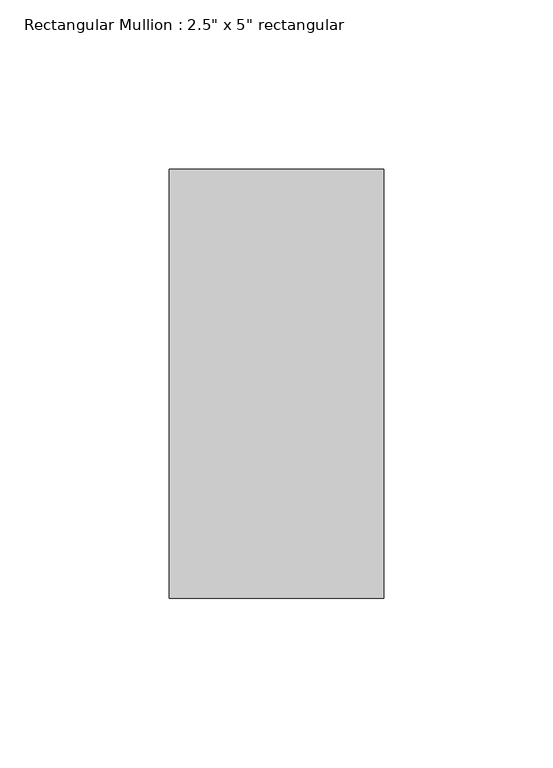
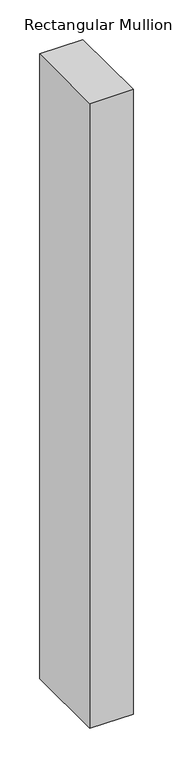
"""IFC4 building model written with IfcOpenShell, lengths in millimetres: member geometry."""

from ifc_helpers import new_model, si_unit, frame, origin, place, context, project, spatial, polyline, outline, extrude, source, transform, mapped, element, save


def member_9193c932(model_context):
    return source(origin(), model_context, "Body", "SweptSolid", [
        extrude(outline(polyline([(0.0, 63.5), (0.0, -63.5), (-63.5, -63.5), (-63.5, 63.5), (0.0, 63.5)])), frame((0.0, 0.0, -965.2), z_axis=(0.0, 0.0, 1.0), x_axis=(1.0, 0.0, 0.0)), (0.0, 0.0, 1.0), 965.2),
    ])


if __name__ == "__main__":
    model = new_model("IFC4")
    model_context = context("Model", 3, world=origin())
    ifc_project = project(units=[si_unit("LENGTHUNIT", "METRE", prefix="MILLI")], contexts=[model_context])
    site = spatial("IfcSite", under=ifc_project)
    building = spatial("IfcBuilding", under=site)
    placement = place(None, origin())
    member_shape = member_9193c932(model_context)
    element("IfcMember", 1, ObjectType="Rectangular Mullion : 2.5\" x 5\" rectangular", at=placement, inside=building, context=model_context, shape_type="MappedRepresentation", body=[
        mapped(member_shape, transform((0.0, 0.0, 0.0), x_axis=(1.0, 0.0, 0.0), y_axis=(0.0, 1.0, 0.0), z_axis=(0.0, 0.0, 1.0))),
    ])
    save(model, "model.ifc")

# Revit data of these elements
# Type "Rectangular Mullion : 2.5\" x 5\" rectangular"
#   built-in parameter 1007304 = 0.416667 (stored number, unit not read)
#   built-in parameter 1007301 = 0.104167 (stored number, unit not read)
#   built-in parameter 1007300 = 0.104167 (stored number, unit not read)
